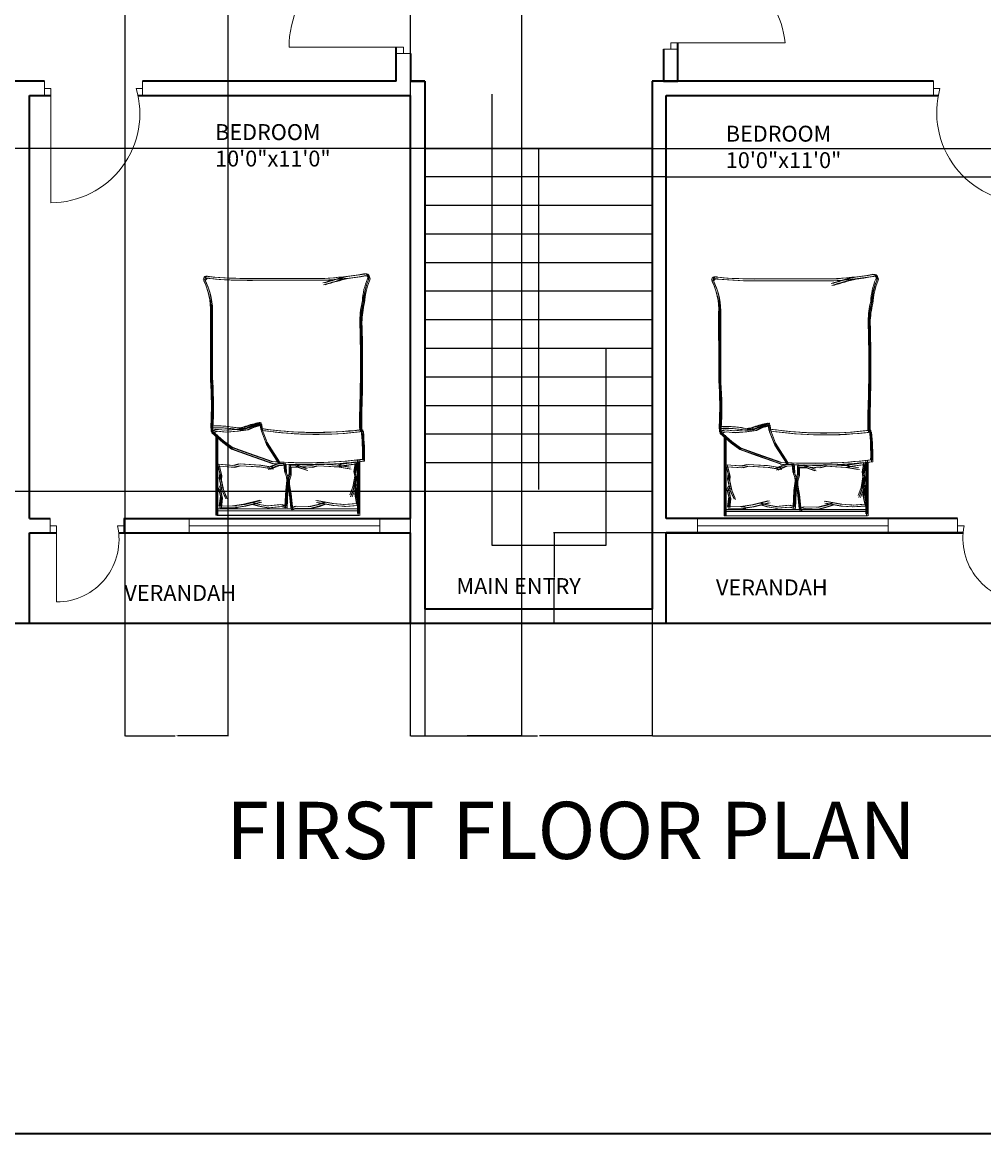
# Model space of a CAD drawing. Units: inches. Extents: x 2234 to 3001, y 1541 to 2386.
# Tile 2 of 12: x 2437 to 2739, y 1541 to 1891. Entities that reach past the tile are written whole.
import ezdxf

# ---------------------------------------------------------------- set-up
doc = ezdxf.new("R2010")
doc.units = ezdxf.units.IN
for name, color, linetype, lineweight in [('A-ANNO-DIMS', 2, 'Continuous', 18), ('A-ANNO-TEXT', 7, 'Continuous', 25), ('A-ANNO-TTLB', 7, 'Continuous', 35), ('A-AREA-IDEN', 7, 'Continuous', 18), ('A-DOOR', 3, 'Continuous', 18), ('A-FLOR-STRS', 7, 'Continuous', 25), ('A-FURN', 9, 'Continuous', 13), ('A-GLAZ', 4, 'Continuous', 18), ('A-WALL', 7, 'Continuous', 35)]:
    doc.layers.add(name, color=color, linetype=linetype, lineweight=lineweight)
doc.styles.get("Standard").update_dxf_attribs({"font": 'arial.ttf'})
doc.dimstyles.get("Standard").update_dxf_attribs({"dimtxt": 0.18, "dimasz": 0.18, "dimexe": 0.18, "dimexo": 0.0625, "dimgap": 0.09, "dimtad": 0, "dimtih": 1, "dimtoh": 1, "dimdec": 4, "dimzin": 0, "dimdsep": 46, "dimtxsty": 'Standard', "dimcen": 0.09, "dimadec": 0, "dimazin": 0, "dimtfac": 1, "dimtdec": 4, "dimtofl": 0, "dimtmove": 0, "dimatfit": 3, "dimfxl": 1, "dimtolj": 1, "dimtzin": 0, "dimarcsym": 0})

# ---------------------------------------------------------------- blocks, each defined once
blk = doc.blocks.new('WIN-60-A')
for p, q in [((0, 60), (4.5, 60)), ((4.5, 60), (2.25, 60)), ((2.25, 60), (2.25, 0)), ((2.25, 0), (0, 0)), ((0, 0), (4.5, 0))]:
    blk.add_line(p, q)
blk = doc.blocks.new('BED-DOUBLE-B')
for p, q in [((37.77, 74.61), (14.78, 74.61)), ((37.77, 74.61), (14.78, 74.61)), ((37.98, 74.02), (15, 74.02)), ((37.98, 74.02), (15, 74.02)), ((38.22, 74.59), (15.24, 74.59)), ((38.22, 74.59), (15.24, 74.59)), ((38.44, 73.99), (15.45, 73.99)), ((38.44, 73.99), (15.46, 73.99)), ((2.39, 28.15), (2.47, 26.53, 3.61)), ((2.39, 28.15), (2.47, 26.53, 3.61)), ((2.85, 28.13), (2.92, 26.5, 3.61)), ((2.85, 28.13), (2.93, 26.5, 3.61)), ((15.47, 28.4), (13.59, 27.54)), ((15.47, 28.4), (13.59, 27.54)), ((15.93, 28.38), (14.05, 27.52)), ((15.93, 28.38), (14.05, 27.52)), ((17.79, 28.98), (15.47, 28.4)), ((17.79, 28.98), (15.47, 28.4)), ((18, 28.38), (15.68, 27.81)), ((18, 28.38), (15.69, 27.81)), ((18.24, 28.96), (15.93, 28.38)), ((18.24, 28.96), (15.93, 28.38)), ((18.46, 28.36), (16.14, 27.79)), ((18.46, 28.36), (16.14, 27.79)), ((18.07, 27.1), (17.79, 28.98)), ((18.07, 27.1), (17.79, 28.98)), ((18.29, 26.51), (18, 28.38)), ((18.29, 26.51), (18, 28.38)), ((18.53, 27.08), (18.24, 28.96)), ((18.53, 27.08), (18.24, 28.96)), ((18.75, 26.49), (18.46, 28.36)), ((18.75, 26.49), (18.46, 28.36)), ((3.9, 27.1), (2.47, 26.53)), ((3.9, 27.1), (2.47, 26.53)), ((2.47, 26.53), (5.93, 23.49)), ((2.47, 26.53), (5.93, 23.49)), ((2.61, 27.56), (2.68, 25.93, 3.61)), ((2.61, 27.56), (2.68, 25.93, 3.61)), ((4.12, 26.51), (2.68, 25.93)), ((4.12, 26.51), (2.68, 25.93)), ((2.68, 25.93), (6.14, 22.89)), ((2.68, 25.93), (6.14, 22.89)), ((4.36, 27.08), (2.92, 26.5)), ((2.92, 26.5), (6.38, 23.47)), ((4.36, 27.08), (2.93, 26.5)), ((2.93, 26.5), (6.39, 23.47)), ((3.06, 27.54), (3.14, 25.91, 3.61)), ((3.06, 27.54), (3.14, 25.91, 3.61)), ((4.57, 26.49), (3.14, 25.91)), ((4.57, 26.49), (3.14, 25.91)), ((3.14, 25.91), (6.6, 22.87)), ((3.14, 25.91), (6.6, 22.87)), ((6.79, 26.81), (3.9, 27.1)), ((6.8, 26.81), (3.9, 27.1)), ((3.96, 0.62), (3.96, 25.46)), ((3.96, 0.62), (3.96, 25.46)), ((7.01, 26.22), (4.12, 26.51)), ((7.01, 26.22), (4.12, 26.51)), ((4.18, 0.02), (4.18, 24.87)), ((4.18, 0.02), (4.18, 24.87)), ((7.25, 26.79), (4.36, 27.08)), ((7.25, 26.79), (4.36, 27.08)), ((4.42, 0.6), (4.42, 25.44)), ((4.42, 0.6), (4.42, 25.44)), ((7.47, 26.2), (4.57, 26.49)), ((7.47, 26.2), (4.57, 26.49)), ((4.63, 0), (4.63, 24.85)), ((4.63, 0), (4.63, 24.85)), ((10.41, 27.1), (6.79, 26.81)), ((10.41, 27.1), (6.8, 26.81)), ((10.62, 26.51), (7.01, 26.22)), ((10.62, 26.51), (7.01, 26.22)), ((10.87, 27.08), (7.25, 26.79)), ((10.87, 27.08), (7.25, 26.79)), ((11.08, 26.49), (7.47, 26.2)), ((11.08, 26.49), (7.47, 26.2)), ((13.59, 27.54), (10.41, 27.1)), ((13.59, 27.54), (10.41, 27.1)), ((13.8, 26.94), (10.62, 26.51)), ((13.81, 26.94), (10.62, 26.51)), ((14.05, 27.52), (10.87, 27.08)), ((14.05, 27.52), (10.87, 27.08)), ((14.26, 26.92), (11.08, 26.49)), ((14.26, 26.92), (11.08, 26.49)), ((15.68, 27.81), (13.8, 26.94)), ((15.69, 27.81), (13.81, 26.94)), ((16.14, 27.79), (14.26, 26.92)), ((16.14, 27.79), (14.26, 26.92)), ((19.67, 22.91), (18.07, 27.1)), ((19.67, 22.91), (18.07, 27.1)), ((19.88, 22.32), (18.29, 26.51)), ((19.88, 22.32), (18.29, 26.51)), ((20.12, 22.89), (18.53, 27.08)), ((20.12, 22.89), (18.53, 27.08)), ((20.34, 22.29), (18.75, 26.49)), ((20.34, 22.29), (18.75, 26.49)), ((5.93, 23.49), (8.67, 21.47)), ((5.93, 23.49), (8.68, 21.47)), ((6.14, 22.89), (8.89, 20.87)), ((6.14, 22.89), (8.89, 20.87)), ((6.38, 23.47), (9.13, 21.45)), ((6.39, 23.47), (9.13, 21.45)), ((6.6, 22.87), (9.35, 20.85)), ((6.6, 22.87), (9.35, 20.85)), ((8.67, 21.47), (13.88, 19.59)), ((8.68, 21.47), (13.88, 19.59)), ((9.13, 21.45), (14.34, 19.57)), ((9.13, 21.45), (14.34, 19.57)), ((23.58, 16.85), (19.67, 22.91)), ((23.58, 16.85), (19.67, 22.91)), ((23.79, 16.25), (19.88, 22.32)), ((23.79, 16.25), (19.88, 22.32)), ((24.04, 16.83), (20.12, 22.89)), ((24.04, 16.83), (20.12, 22.89)), ((24.25, 16.23), (20.34, 22.29)), ((24.25, 16.23), (20.34, 22.29)), ((8.89, 20.87), (14.09, 18.99)), ((8.89, 20.87), (14.09, 18.99)), ((9.35, 20.85), (14.55, 18.97)), ((9.35, 20.85), (14.55, 18.97)), ((13.88, 19.59), (21.67, 16.85)), ((13.88, 19.59), (21.67, 16.85)), ((14.09, 18.99), (21.88, 16.25)), ((14.09, 18.99), (21.88, 16.25)), ((14.34, 19.57), (22.12, 16.83)), ((14.34, 19.57), (22.12, 16.83)), ((14.55, 18.97), (22.34, 16.23)), ((14.55, 18.97), (22.34, 16.23)), ((48.59, 17.53), (48.59, 0.62)), ((48.59, 17.53), (48.59, 0.62)), ((49.05, 17.51), (49.05, 0.6)), ((49.05, 17.51), (49.05, 0.6)), ((9.28, 15.72), (4.49, 16.09)), ((4.49, 16.09), (5.22, 13.16)), ((9.29, 15.72), (4.49, 16.09)), ((4.49, 16.09), (5.22, 13.16)), ((9.5, 15.12), (4.71, 15.5)), ((4.71, 15.5), (5.43, 12.56)), ((9.5, 15.12), (4.71, 15.5)), ((4.71, 15.5), (5.43, 12.56)), ((9.74, 15.69), (4.95, 16.07)), ((4.95, 16.07), (5.67, 13.14)), ((9.74, 15.69), (4.95, 16.07)), ((4.95, 16.07), (5.67, 13.14)), ((9.96, 15.1), (5.16, 15.47)), ((5.16, 15.47), (5.89, 12.54)), ((9.96, 15.1), (5.16, 15.47)), ((5.16, 15.47), (5.89, 12.54)), ((11.12, 16.24), (9.28, 15.72)), ((11.12, 16.24), (9.29, 15.72)), ((11.33, 15.64), (9.5, 15.12)), ((11.33, 15.64), (9.5, 15.12)), ((11.57, 16.21), (9.74, 15.69)), ((11.57, 16.21), (9.74, 15.69)), ((11.79, 15.62), (9.96, 15.1)), ((11.79, 15.62), (9.96, 15.1)), ((17.66, 15.83), (11.12, 16.24)), ((17.66, 15.83), (11.12, 16.24)), ((17.87, 15.24), (11.33, 15.64)), ((17.87, 15.24), (11.33, 15.64)), ((18.12, 15.81), (11.57, 16.21)), ((18.12, 15.81), (11.57, 16.21)), ((18.33, 15.22), (11.79, 15.62)), ((18.33, 15.22), (11.79, 15.62)), ((21.43, 15.21), (17.66, 15.83)), ((21.43, 15.21), (17.66, 15.83)), ((21.64, 14.61), (17.87, 15.24)), ((21.64, 14.61), (17.87, 15.24)), ((21.88, 15.19), (18.12, 15.81)), ((21.88, 15.19), (18.12, 15.81)), ((22.1, 14.59), (18.33, 15.22)), ((22.1, 14.59), (18.33, 15.22)), ((23.12, 16.25), (20.25, 15.05)), ((23.12, 16.25), (20.25, 15.05)), ((23.33, 15.65), (20.47, 14.45)), ((23.33, 15.65), (20.47, 14.45)), ((23.58, 16.23), (20.71, 15.03)), ((23.58, 16.23), (20.71, 15.03)), ((23.79, 15.63), (20.92, 14.43)), ((23.79, 15.63), (20.92, 14.43)), ((25.41, 16.39), (23.12, 16.25)), ((25.41, 16.39), (23.12, 16.25)), ((25.62, 15.79), (23.33, 15.65)), ((25.62, 15.79), (23.33, 15.65)), ((25.87, 16.37), (23.58, 16.23)), ((25.87, 16.37), (23.58, 16.23)), ((26.08, 15.77), (23.79, 15.63)), ((26.08, 15.77), (23.79, 15.63)), ((25.57, 13.89), (25.41, 16.39)), ((25.57, 13.89), (25.41, 16.39)), ((25.78, 13.3), (25.62, 15.79)), ((25.78, 13.3), (25.62, 15.79)), ((26.02, 13.87), (25.87, 16.37)), ((26.02, 13.87), (25.87, 16.37)), ((26.24, 13.27), (26.08, 15.77)), ((26.24, 13.27), (26.08, 15.77)), ((27.03, 13.3), (27.03, 15.8)), ((27.03, 15.8), (29.33, 15.8)), ((27.03, 13.3), (27.03, 15.8)), ((27.03, 15.8), (29.33, 15.8)), ((27.24, 12.7), (27.24, 15.21)), ((27.24, 15.21), (29.54, 15.21)), ((27.24, 12.7), (27.24, 15.21)), ((27.24, 15.21), (29.54, 15.21)), ((27.49, 13.28), (27.49, 15.78)), ((27.49, 15.78), (29.78, 15.78)), ((27.49, 13.28), (27.49, 15.78)), ((27.49, 15.78), (29.78, 15.78)), ((27.7, 12.68), (27.7, 15.19)), ((27.7, 15.19), (30, 15.19)), ((27.7, 12.68), (27.7, 15.19)), ((27.7, 15.19), (30, 15.19)), ((33.73, 15.72), (28.94, 16.09)), ((33.73, 15.72), (28.94, 16.09)), ((33.95, 15.12), (29.15, 15.5)), ((33.95, 15.12), (29.15, 15.5)), ((29.33, 15.8), (32.26, 14.78)), ((29.33, 15.8), (32.26, 14.78)), ((34.19, 15.69), (29.4, 16.07)), ((34.19, 15.69), (29.4, 16.07)), ((29.54, 15.21), (32.48, 14.19)), ((29.54, 15.21), (32.48, 14.19)), ((34.4, 15.1), (29.61, 15.47)), ((34.4, 15.1), (29.61, 15.47)), ((29.78, 15.78), (32.72, 14.76)), ((29.78, 15.78), (32.72, 14.76)), ((30, 15.19), (32.93, 14.17)), ((30, 15.19), (32.93, 14.17)), ((35.56, 16.24), (33.73, 15.72)), ((35.56, 16.24), (33.73, 15.72)), ((35.78, 15.64), (33.95, 15.12)), ((35.78, 15.64), (33.95, 15.12)), ((36.02, 16.21), (34.19, 15.69)), ((36.02, 16.21), (34.19, 15.69)), ((36.23, 15.62), (34.4, 15.1)), ((36.23, 15.62), (34.4, 15.1)), ((42.11, 15.83), (35.56, 16.24)), ((42.11, 15.83), (35.56, 16.24)), ((42.32, 15.24), (35.78, 15.64)), ((42.32, 15.24), (35.78, 15.64)), ((42.57, 15.81), (36.02, 16.21)), ((42.57, 15.81), (36.02, 16.21)), ((42.78, 15.22), (36.23, 15.62)), ((42.78, 15.22), (36.23, 15.62)), ((42.11, 15.83), (43.17, 16.13)), ((42.11, 15.83), (43.17, 16.13)), ((45.87, 15.21), (42.11, 15.83)), ((45.87, 15.21), (42.11, 15.83)), ((42.32, 15.24), (43.38, 15.54)), ((42.32, 15.24), (43.38, 15.54)), ((46.09, 14.61), (42.32, 15.24)), ((46.09, 14.61), (42.32, 15.24)), ((42.57, 15.81), (43.62, 16.11)), ((42.57, 15.81), (43.62, 16.11)), ((46.33, 15.19), (42.57, 15.81)), ((46.33, 15.19), (42.57, 15.81)), ((42.78, 15.22), (43.84, 15.52)), ((42.78, 15.22), (43.84, 15.52)), ((46.54, 14.59), (42.78, 15.22)), ((46.54, 14.59), (42.78, 15.22)), ((43.17, 16.13), (47.93, 16.81)), ((43.17, 16.13), (47.93, 16.81)), ((43.38, 15.54), (48.14, 16.21)), ((43.38, 15.54), (48.14, 16.21)), ((43.62, 16.11), (48.38, 16.79)), ((43.62, 16.11), (48.38, 16.79)), ((43.84, 15.52), (48.6, 16.19)), ((43.84, 15.52), (48.6, 16.19)), ((47.93, 16.81), (47.39, 13.84)), ((47.93, 16.81), (47.39, 13.84)), ((48.14, 16.21), (47.6, 13.24)), ((48.14, 16.21), (47.6, 13.24)), ((48.38, 16.79), (47.84, 13.82)), ((48.38, 16.79), (47.84, 13.82)), ((48.6, 16.19), (48.06, 13.22)), ((48.6, 16.19), (48.06, 13.22)), ((48.8, 16.93), (48.8, 0.02)), ((48.8, 16.93), (48.8, 0.02)), ((49.26, 16.91), (49.26, 0)), ((49.26, 16.91), (49.26, 0)), ((5.22, 13.16), (5.04, 11.66)), ((5.22, 13.16), (5.04, 11.66)), ((5.04, 11.66), (5.79, 8.33)), ((5.04, 11.66), (5.79, 8.33)), ((5.43, 12.56), (5.25, 11.07)), ((5.43, 12.56), (5.25, 11.07)), ((5.25, 11.07), (6, 7.73)), ((5.25, 11.07), (6, 7.73)), ((5.67, 13.14), (5.5, 11.64)), ((5.67, 13.14), (5.5, 11.64)), ((5.5, 11.64), (6.25, 8.31)), ((5.5, 11.64), (6.25, 8.31)), ((5.89, 12.54), (5.71, 11.04)), ((5.89, 12.54), (5.71, 11.04)), ((5.71, 11.04), (6.46, 7.71)), ((5.71, 11.04), (6.46, 7.71)), ((26.21, 12.17), (25.57, 13.89)), ((26.21, 12.17), (25.57, 13.89)), ((26.43, 11.58), (25.78, 13.3)), ((26.43, 11.58), (25.78, 13.3)), ((25.94, 7.96), (26.29, 10.96)), ((25.94, 7.96), (26.29, 10.96)), ((26.67, 12.15), (26.02, 13.87)), ((26.67, 12.15), (26.02, 13.87)), ((26.29, 10.96), (26.21, 12.17)), ((26.29, 10.96), (26.21, 12.17)), ((26.88, 11.56), (26.24, 13.27)), ((26.89, 11.56), (26.24, 13.27)), ((26.39, 7.94), (26.75, 10.94)), ((26.39, 7.94), (26.75, 10.94)), ((26.5, 10.36), (26.43, 11.58)), ((26.5, 10.36), (26.43, 11.58)), ((26.49, 11.54), (27.03, 13.3)), ((26.49, 11.54), (27.03, 13.3)), ((26.49, 10.33), (26.49, 11.54)), ((26.49, 10.33), (26.49, 11.54)), ((26.75, 10.94), (26.67, 12.15)), ((26.75, 10.94), (26.67, 12.15)), ((26.7, 10.95), (27.24, 12.7)), ((26.7, 10.95), (27.24, 12.7)), ((26.7, 9.73), (26.7, 10.95)), ((26.7, 9.73), (26.7, 10.95)), ((26.96, 10.34), (26.88, 11.56)), ((26.96, 10.34), (26.89, 11.56)), ((26.95, 11.52), (27.49, 13.28)), ((26.95, 11.52), (27.49, 13.28)), ((26.95, 10.31), (26.95, 11.52)), ((26.95, 10.31), (26.95, 11.52)), ((27.16, 10.93), (27.7, 12.68)), ((27.16, 10.93), (27.7, 12.68)), ((27.16, 9.71), (27.16, 10.93)), ((27.16, 9.71), (27.16, 10.93)), ((47.66, 12.35), (47.12, 8.98)), ((47.66, 12.35), (47.12, 8.98)), ((47.87, 11.76), (47.33, 8.38)), ((47.87, 11.76), (47.33, 8.38)), ((47.39, 13.84), (47.66, 12.35)), ((47.39, 13.84), (47.66, 12.35)), ((48.11, 12.33), (47.57, 8.96)), ((48.11, 12.33), (47.57, 8.96)), ((47.6, 13.24), (47.87, 11.76)), ((47.6, 13.24), (47.87, 11.76)), ((48.33, 11.74), (47.79, 8.36)), ((48.33, 11.74), (47.79, 8.36)), ((47.84, 13.82), (48.11, 12.33)), ((47.84, 13.82), (48.11, 12.33)), ((48.06, 13.22), (48.33, 11.74)), ((48.06, 13.22), (48.33, 11.74)), ((4.84, 8.4), (5.32, 9.38)), ((4.84, 8.4), (5.32, 9.38)), ((5.39, 6), (4.84, 8.4)), ((5.39, 6), (4.84, 8.4)), ((5.05, 7.81), (5.53, 8.78)), ((5.05, 7.81), (5.53, 8.78)), ((5.61, 5.41), (5.05, 7.81)), ((5.61, 5.41), (5.05, 7.81)), ((5.3, 8.38), (5.78, 9.36)), ((5.3, 8.38), (5.78, 9.36)), ((5.85, 5.98), (5.3, 8.38)), ((5.85, 5.98), (5.3, 8.38)), ((5.51, 7.79), (5.99, 8.76)), ((5.51, 7.79), (5.99, 8.76)), ((6.06, 5.39), (5.51, 7.79)), ((6.07, 5.39), (5.51, 7.79)), ((5.79, 8.33), (6.89, 5.83)), ((5.79, 8.33), (6.89, 5.83)), ((6, 7.73), (7.11, 5.23)), ((6, 7.73), (7.11, 5.23)), ((6.25, 8.31), (7.35, 5.81)), ((6.25, 8.31), (7.35, 5.81)), ((6.46, 7.71), (7.56, 5.21)), ((6.46, 7.71), (7.56, 5.21)), ((25.71, 2.94), (25.94, 7.96)), ((25.71, 2.94), (25.94, 7.96)), ((25.92, 2.35), (26.15, 7.37)), ((25.92, 2.35), (26.15, 7.37)), ((26.15, 7.37), (26.5, 10.36)), ((26.15, 7.37), (26.5, 10.36)), ((26.17, 2.92), (26.39, 7.94)), ((26.17, 2.92), (26.39, 7.94)), ((26.38, 2.33), (26.61, 7.35)), ((26.38, 2.33), (26.61, 7.35)), ((27.03, 7.36), (26.49, 10.33)), ((27.03, 7.36), (26.49, 10.33)), ((26.61, 7.35), (26.96, 10.34)), ((26.61, 7.35), (26.96, 10.34)), ((27.24, 6.76), (26.7, 9.73)), ((27.24, 6.76), (26.7, 9.73)), ((27.49, 7.34), (26.95, 10.31)), ((27.49, 7.34), (26.95, 10.31)), ((27.57, 2.36), (27.03, 7.36)), ((27.57, 2.36), (27.03, 7.36)), ((27.7, 6.74), (27.16, 9.71)), ((27.7, 6.74), (27.16, 9.71)), ((28.03, 2.34), (27.49, 7.34)), ((28.03, 2.34), (27.49, 7.34)), ((47.12, 8.98), (46.17, 6.41)), ((47.12, 8.98), (46.17, 6.41)), ((47.33, 8.38), (46.38, 5.82)), ((47.33, 8.38), (46.38, 5.82)), ((47.57, 8.96), (46.63, 6.39)), ((47.57, 8.96), (46.63, 6.39)), ((47.79, 8.36), (46.84, 5.8)), ((47.79, 8.36), (46.84, 5.8)), ((48.06, 9.11), (47.52, 10.06)), ((48.06, 9.11), (47.52, 10.06)), ((47.66, 6.68), (48.06, 9.11)), ((47.66, 6.68), (48.06, 9.11)), ((48.27, 8.52), (47.73, 9.46)), ((48.27, 8.52), (47.73, 9.46)), ((47.87, 6.09), (48.27, 8.52)), ((47.87, 6.09), (48.27, 8.52)), ((48.52, 9.09), (47.98, 10.04)), ((48.52, 9.09), (47.98, 10.04)), ((48.11, 6.66), (48.52, 9.09)), ((48.11, 6.66), (48.52, 9.09)), ((48.73, 8.5), (48.19, 9.44)), ((48.73, 8.5), (48.19, 9.44)), ((48.33, 6.07), (48.73, 8.5)), ((48.33, 6.07), (48.73, 8.5)), ((5.04, 3.01), (5.39, 6)), ((5.04, 3.01), (5.39, 6)), ((5.25, 2.41), (5.61, 5.41)), ((5.25, 2.41), (5.61, 5.41)), ((5.5, 2.98), (5.85, 5.98)), ((5.5, 2.98), (5.85, 5.98)), ((5.71, 2.39), (6.06, 5.39)), ((5.71, 2.39), (6.07, 5.39)), ((12.69, 3.48), (17.76, 4.75)), ((12.7, 3.48), (17.76, 4.75)), ((12.91, 2.89), (17.97, 4.15)), ((12.91, 2.89), (17.97, 4.15)), ((13.15, 3.46), (18.21, 4.73)), ((13.15, 3.46), (18.21, 4.73)), ((13.37, 2.87), (18.43, 4.13)), ((13.37, 2.87), (18.43, 4.13)), ((15.23, 4.05), (17.16, 3.49)), ((15.23, 4.05), (17.16, 3.49)), ((15.69, 4.03), (17.61, 3.47)), ((15.69, 4.03), (17.62, 3.47)), ((27.78, 1.77), (27.24, 6.76)), ((27.78, 1.77), (27.24, 6.76)), ((28.24, 1.75), (27.7, 6.74)), ((28.24, 1.75), (27.7, 6.74)), ((40.53, 3.71), (35.4, 4.66)), ((40.53, 3.71), (35.4, 4.66)), ((40.74, 3.12), (35.61, 4.06)), ((40.74, 3.12), (35.61, 4.06)), ((40.98, 3.69), (35.85, 4.64)), ((40.98, 3.69), (35.85, 4.64)), ((37.96, 4.12), (36.07, 3.44)), ((37.96, 4.12), (36.07, 3.44)), ((41.2, 3.1), (36.07, 4.04)), ((41.2, 3.1), (36.07, 4.04)), ((38.17, 3.52), (36.29, 2.85)), ((38.18, 3.52), (36.29, 2.85)), ((38.42, 4.1), (36.53, 3.42)), ((38.42, 4.1), (36.53, 3.42)), ((38.63, 3.5), (36.74, 2.83)), ((38.63, 3.5), (36.74, 2.83)), ((44.1, 3.44), (40.53, 3.71)), ((44.1, 3.44), (40.53, 3.71)), ((44.55, 3.42), (40.98, 3.69)), ((44.55, 3.42), (40.98, 3.69)), ((48.19, 3.73), (44.19, 3.43)), ((48.19, 3.73), (44.2, 3.43)), ((48.65, 3.71), (44.65, 3.41)), ((48.65, 3.71), (44.65, 3.41)), ((48.2, 3.71), (47.66, 6.68)), ((48.2, 3.71), (47.66, 6.68)), ((48.41, 3.12), (47.87, 6.09)), ((48.41, 3.12), (47.87, 6.09)), ((48.65, 3.69), (48.11, 6.66)), ((48.65, 3.69), (48.11, 6.66)), ((48.87, 3.1), (48.33, 6.07)), ((48.87, 3.1), (48.33, 6.07)), ((48.59, 2.05), (3.96, 2.05)), ((48.59, 2.05), (3.96, 2.05)), ((3.96, 0.02), (3.96, 0.62)), ((3.96, 0.02), (48.59, 0.02)), ((48.8, 1.45), (4.18, 1.45)), ((48.8, 1.45), (4.18, 1.45)), ((49.05, 2.03), (4.42, 2.03)), ((49.05, 2.03), (4.42, 2.03)), ((4.42, 0), (4.42, 0.6)), ((49.26, 1.43), (4.63, 1.43)), ((49.26, 1.43), (4.63, 1.43)), ((5.04, 3.01), (10.08, 2.91)), ((5.04, 3.01), (10.09, 2.91)), ((5.25, 2.41), (10.3, 2.32)), ((5.25, 2.41), (10.3, 2.32)), ((5.5, 2.98), (10.54, 2.89)), ((5.5, 2.98), (10.54, 2.89)), ((5.71, 2.39), (10.76, 2.3)), ((5.71, 2.39), (10.76, 2.3)), ((9.15, 2.99), (12.69, 3.48)), ((9.15, 2.99), (12.7, 3.48)), ((10.08, 2.91), (9.15, 2.99)), ((10.09, 2.91), (9.15, 2.99)), ((9.36, 2.39), (12.91, 2.89)), ((9.36, 2.39), (12.91, 2.89)), ((10.3, 2.32), (9.36, 2.39)), ((10.3, 2.32), (9.36, 2.39)), ((9.61, 2.97), (13.15, 3.46)), ((9.61, 2.97), (13.15, 3.46)), ((10.54, 2.89), (9.61, 2.97)), ((10.54, 2.89), (9.61, 2.97)), ((9.82, 2.37), (13.37, 2.87)), ((9.82, 2.37), (13.37, 2.87)), ((10.76, 2.3), (9.82, 2.37)), ((10.76, 2.3), (9.82, 2.37)), ((15.44, 3.45), (17.37, 2.89)), ((15.44, 3.45), (17.37, 2.89)), ((15.9, 3.43), (17.83, 2.87)), ((15.9, 3.43), (17.83, 2.87)), ((17.16, 3.49), (19.89, 2.99)), ((17.16, 3.49), (19.89, 2.99)), ((17.37, 2.89), (20.11, 2.39)), ((17.37, 2.89), (20.11, 2.39)), ((17.61, 3.47), (20.35, 2.97)), ((17.62, 3.47), (20.35, 2.97)), ((17.83, 2.87), (20.56, 2.37)), ((17.83, 2.87), (20.56, 2.37)), ((19.89, 2.99), (20.19, 3.01)), ((19.89, 2.99), (20.19, 3.01)), ((20.11, 2.39), (20.41, 2.41)), ((20.11, 2.39), (20.41, 2.41)), ((20.19, 3.01), (24.33, 3.4)), ((20.19, 3.01), (24.33, 3.4)), ((20.35, 2.97), (20.65, 2.98)), ((20.35, 2.97), (20.65, 2.98)), ((20.41, 2.41), (24.54, 2.8)), ((20.41, 2.41), (24.54, 2.8)), ((20.56, 2.37), (20.86, 2.39)), ((20.56, 2.37), (20.86, 2.39)), ((20.65, 2.98), (24.79, 3.38)), ((20.65, 2.98), (24.79, 3.38)), ((20.86, 2.39), (25, 2.78)), ((20.86, 2.39), (25, 2.78)), ((24.33, 3.4), (25.71, 2.94)), ((24.33, 3.4), (25.71, 2.94)), ((24.54, 2.8), (25.92, 2.35)), ((24.54, 2.8), (25.92, 2.35)), ((24.79, 3.38), (26.17, 2.92)), ((24.79, 3.38), (26.17, 2.92)), ((25, 2.78), (26.38, 2.33)), ((25, 2.78), (26.38, 2.33)), ((28.92, 2.9), (27.57, 2.36)), ((28.92, 2.9), (27.57, 2.36)), ((29.13, 2.31), (27.78, 1.77)), ((29.13, 2.31), (27.78, 1.77)), ((29.38, 2.88), (28.03, 2.34)), ((29.38, 2.88), (28.03, 2.34)), ((29.59, 2.29), (28.24, 1.75)), ((29.59, 2.29), (28.24, 1.75)), ((33.07, 2.77), (28.92, 2.9)), ((33.07, 2.77), (28.92, 2.9)), ((33.29, 2.17), (29.13, 2.31)), ((33.29, 2.17), (29.13, 2.31)), ((33.53, 2.75), (29.38, 2.88)), ((33.53, 2.75), (29.38, 2.88)), ((33.74, 2.15), (29.59, 2.29)), ((33.74, 2.15), (29.59, 2.29)), ((33.37, 2.77), (33.07, 2.77)), ((33.37, 2.77), (33.07, 2.77)), ((33.59, 2.17), (33.29, 2.17)), ((33.59, 2.17), (33.29, 2.17)), ((36.07, 3.44), (33.37, 2.77)), ((36.07, 3.44), (33.37, 2.77)), ((33.83, 2.75), (33.53, 2.75)), ((33.83, 2.75), (33.53, 2.75)), ((36.29, 2.85), (33.59, 2.17)), ((36.29, 2.85), (33.59, 2.17)), ((34.04, 2.15), (33.74, 2.15)), ((34.04, 2.15), (33.74, 2.15)), ((36.53, 3.42), (33.83, 2.75)), ((36.53, 3.42), (33.83, 2.75)), ((36.74, 2.83), (34.04, 2.15)), ((36.74, 2.83), (34.04, 2.15)), ((44.31, 2.85), (40.74, 3.12)), ((44.31, 2.85), (40.74, 3.12)), ((44.77, 2.83), (41.2, 3.1)), ((44.77, 2.83), (41.2, 3.1)), ((44.19, 3.43), (44.1, 3.44)), ((44.2, 3.43), (44.1, 3.44)), ((44.41, 2.83), (44.31, 2.85)), ((44.41, 2.83), (44.31, 2.85)), ((48.41, 3.14), (44.41, 2.83)), ((48.41, 3.14), (44.41, 2.83)), ((44.65, 3.41), (44.55, 3.42)), ((44.65, 3.41), (44.55, 3.42)), ((44.87, 2.81), (44.77, 2.83)), ((44.87, 2.81), (44.77, 2.83)), ((48.86, 3.12), (44.87, 2.81)), ((48.86, 3.12), (44.87, 2.81)), ((4.42, 0), (49.05, 0))]:
    blk.add_line(p, q)
for centre, radius, start, end in [((1.03, 74.26), 1.03, 62.6588, 176.02), ((1.03, 74.26), 1.03, 62.6588, 176.02), ((-19.28, 64.73), 21.54, 357.4714, 26.4681), ((-19.28, 64.73), 21.54, 357.4714, 26.4681), ((1.24, 73.67), 1.03, 62.6588, 176.02), ((1.24, 73.67), 1.03, 62.6588, 176.02), ((-19.07, 64.14), 21.54, 357.4714, 26.4681), ((-19.07, 64.14), 21.54, 357.4714, 26.4681), ((1.48, 74.24), 1.03, 62.6588, 176.02), ((1.49, 74.24), 1.03, 62.6588, 176.02), ((-18.82, 64.71), 21.54, 357.4714, 26.4681), ((-18.82, 64.71), 21.54, 357.4714, 26.4681), ((1.7, 73.64), 1.03, 62.6588, 176.02), ((1.7, 73.64), 1.03, 62.6588, 176.02), ((-18.61, 64.12), 21.54, 357.4714, 26.4681), ((-18.61, 64.12), 21.54, 357.4714, 26.4681), ((13.41, 198.83), 124.23, 264.4998, 270.6351), ((13.41, 198.83), 124.23, 264.4998, 270.6351), ((13.62, 198.23), 124.23, 264.4998, 270.6351), ((13.62, 198.23), 124.23, 264.4998, 270.6351), ((13.86, 198.81), 124.23, 264.4998, 270.6351), ((13.86, 198.81), 124.23, 264.4998, 270.6351), ((14.08, 198.21), 124.23, 264.4998, 270.6351), ((14.08, 198.21), 124.23, 264.4998, 270.6351), ((67.91, -21.52), 99.41, 103.3832, 107.7053), ((67.91, -21.52), 99.41, 103.3832, 107.7053), ((31.83, 188.15), 113.69, 272.9958, 279.4091), ((31.83, 188.15), 113.69, 272.9958, 279.4091), ((68.13, -22.12), 99.41, 103.3832, 107.7053), ((68.13, -22.12), 99.41, 103.3832, 107.7053), ((32.04, 187.55), 113.69, 272.9958, 279.4091), ((32.04, 187.55), 113.69, 272.9958, 279.4091), ((68.37, -21.54), 99.41, 103.3832, 107.7053), ((68.37, -21.54), 99.41, 103.3832, 107.7053), ((32.28, 188.13), 113.69, 272.9958, 279.4091), ((32.28, 188.13), 113.69, 272.9958, 279.4091), ((68.58, -22.14), 99.41, 103.3832, 107.7053), ((68.58, -22.14), 99.41, 103.3832, 107.7053), ((32.5, 187.53), 113.69, 272.9958, 279.4091), ((32.5, 187.53), 113.69, 272.9958, 279.4091), ((72.06, 66.24), 22, 157.9751, 176.652), ((72.06, 66.24), 22, 157.9751, 176.652), ((72.27, 65.64), 22, 157.9751, 176.652), ((72.27, 65.64), 22, 157.9751, 176.652), ((50.82, 75.05), 1.02, 326.1736, 113.4781), ((50.82, 75.05), 1.02, 326.1736, 113.4781), ((72.51, 66.22), 22, 157.9751, 176.652), ((72.51, 66.22), 22, 157.9751, 176.652), ((51.03, 74.46), 1.02, 326.1736, 113.4781), ((51.03, 74.46), 1.02, 326.1736, 113.4781), ((72.73, 65.62), 22, 157.9751, 176.652), ((72.73, 65.62), 22, 157.9751, 176.652), ((51.27, 75.03), 1.02, 326.1736, 113.4781), ((51.27, 75.03), 1.02, 326.1736, 113.4781), ((51.49, 74.44), 1.02, 326.1736, 113.4781), ((51.49, 74.44), 1.02, 326.1736, 113.4781), ((76.95, 60.86), 27.67, 166.0648, 178.9113), ((76.95, 60.86), 27.67, 166.0648, 178.9113), ((77.16, 60.26), 27.67, 166.0648, 178.9113), ((77.16, 60.26), 27.67, 166.0648, 178.9113), ((77.41, 60.84), 27.67, 166.0648, 178.9113), ((77.41, 60.84), 27.67, 166.0648, 178.9113), ((77.62, 60.24), 27.67, 166.0648, 178.9113), ((77.62, 60.24), 27.67, 166.0648, 178.9113), ((4261.85, 63.95), 4259.62, 180.00217, 180.28689), ((4261.85, 63.95), 4259.62, 180.00217, 180.28689), ((4262.07, 63.35), 4259.62, 180.00217, 180.28689), ((4262.07, 63.35), 4259.62, 180.00217, 180.28689), ((4262.31, 63.92), 4259.62, 180.00217, 180.28689), ((4262.31, 63.92), 4259.62, 180.00217, 180.28689), ((4262.53, 63.33), 4259.62, 180.00217, 180.28689), ((4262.53, 63.33), 4259.62, 180.00217, 180.28689), ((-400.87, 47.88), 450.36, 358.2277, 1.7185), ((-400.87, 47.88), 450.36, 358.2277, 1.7185), ((-400.66, 47.28), 450.36, 358.2277, 1.7185), ((-400.66, 47.28), 450.36, 358.2277, 1.7185), ((-400.41, 47.86), 450.36, 358.2277, 1.7185), ((-400.41, 47.86), 450.36, 358.2277, 1.7185), ((-400.2, 47.26), 450.36, 358.2277, 1.7185), ((-400.2, 47.26), 450.36, 358.2277, 1.7185), ((-118.36, 34.53), 120.92, 356.9791, 3.8365), ((-118.36, 34.53), 120.92, 356.9791, 3.8365), ((-118.14, 33.93), 120.92, 356.9791, 3.8365), ((-118.14, 33.93), 120.92, 356.9791, 3.8365), ((-117.9, 34.51), 120.92, 356.9791, 3.8365), ((-117.9, 34.51), 120.92, 356.9791, 3.8365), ((-117.69, 33.91), 120.92, 356.9791, 3.8365), ((-117.69, 33.91), 120.92, 356.9791, 3.8365), ((208.05, 29.73), 158.84, 178.4762, 181.0082), ((208.06, 29.73), 158.84, 178.4762, 181.0082), ((208.27, 29.13), 158.84, 178.4762, 181.0082), ((208.27, 29.13), 158.84, 178.4762, 181.0082), ((208.51, 29.7), 158.84, 178.4762, 181.0082), ((208.51, 29.7), 158.84, 178.4762, 181.0082), ((208.73, 29.11), 158.84, 178.4762, 181.0082), ((208.73, 29.11), 158.84, 178.4762, 181.0082), ((3.91, -5.6), 33.79, 79.8763, 92.5657), ((3.91, -5.6), 33.79, 79.8763, 92.5657), ((4.36, -5.62), 33.79, 79.8763, 92.5657), ((4.36, -5.62), 33.79, 79.8763, 92.5657), ((10.99, 33.36), 5.81, 258.6608, 293.7384), ((10.99, 33.36), 5.81, 258.6608, 293.7384), ((11.44, 33.34), 5.81, 258.6608, 293.7384), ((11.44, 33.34), 5.81, 258.6608, 293.7384), ((22.74, 2), 27.69, 100.6617, 109.8806), ((22.74, 2), 27.69, 100.6617, 109.8806), ((22.96, 1.4), 27.69, 100.6617, 109.8806), ((22.96, 1.4), 27.69, 100.6617, 109.8806), ((23.2, 1.98), 27.69, 100.6617, 109.8806), ((23.2, 1.98), 27.69, 100.6617, 109.8806), ((23.41, 1.38), 27.69, 100.6617, 109.8806), ((23.41, 1.38), 27.69, 100.6617, 109.8806), ((17.62, 29.04), 0.172, 340.2464, 91.1377), ((17.62, 29.04), 0.172, 340.2464, 91.1377), ((17.84, 28.44), 0.172, 340.2464, 91.1377), ((17.84, 28.44), 0.172, 340.2464, 91.1377), ((18.08, 29.02), 0.172, 340.2464, 91.1377), ((18.08, 29.02), 0.172, 340.2464, 91.1377), ((18.29, 28.42), 0.172, 340.2464, 91.1377), ((18.29, 28.42), 0.172, 340.2464, 91.1377), ((4.12, -6.19), 33.79, 79.8763, 92.5657), ((4.12, -6.19), 33.79, 79.8763, 92.5657), ((4.58, -6.22), 33.79, 79.8763, 92.5657), ((4.58, -6.22), 33.79, 79.8763, 92.5657), ((11.2, 32.76), 5.81, 258.6608, 293.7384), ((11.2, 32.76), 5.81, 258.6608, 293.7384), ((11.66, 32.74), 5.81, 258.6608, 293.7384), ((11.66, 32.74), 5.81, 258.6608, 293.7384), ((35.25, 146.58), 120.47, 261.7845, 276.9006), ((35.25, 146.58), 120.47, 261.7845, 276.9006), ((35.47, 145.98), 120.47, 261.7845, 276.9006), ((35.47, 145.98), 120.47, 261.7845, 276.9006), ((35.71, 146.56), 120.47, 261.7845, 276.9006), ((35.71, 146.56), 120.47, 261.7845, 276.9006), ((35.92, 145.96), 120.47, 261.7845, 276.9006), ((35.92, 145.96), 120.47, 261.7845, 276.9006), ((-27.69, 19.38), 77.79, 358.7218, 5.604), ((-27.69, 19.38), 77.79, 358.7218, 5.604), ((-27.47, 18.79), 77.79, 358.7218, 5.604), ((-27.47, 18.79), 77.79, 358.7218, 5.604), ((-27.23, 19.36), 77.79, 358.7218, 5.604), ((-27.23, 19.36), 77.79, 358.7218, 5.604), ((-27.02, 18.76), 77.79, 358.7218, 5.604), ((-27.02, 18.76), 77.79, 358.7218, 5.604), ((31.89, 170.61), 154.04, 266.0865, 276.7821), ((31.89, 170.61), 154.04, 266.0865, 276.7821), ((32.35, 170.59), 154.04, 266.0865, 276.7821), ((32.35, 170.59), 154.04, 266.0865, 276.7821), ((32.1, 170.01), 154.04, 266.0865, 276.7821), ((32.1, 170.01), 154.04, 266.0865, 276.7821), ((32.56, 169.99), 154.04, 266.0865, 276.7821), ((32.56, 169.99), 154.04, 266.0865, 276.7821)]:
    blk.add_arc(centre, radius, start, end)
blk = doc.blocks.new('*D64')
at = {"layer": 'A-ANNO-DIMS', "color": 0, "lineweight": -2, "transparency": 16777216}
for p, q in [((2563.25, 1706.55), (2563.25, 1666.58)), ((2634.75, 1706.55), (2634.75, 1666.58)), ((2563.43, 1666.76), (2598.68, 1666.76)), ((2634.57, 1666.76), (2599.33, 1666.76))]:
    blk.add_line(p, q, dxfattribs=at)
at = {"layer": 'A-ANNO-DIMS', "color": 0, "transparency": 16777216}
for points in [[(2563.43, 1666.79), (2563.43, 1666.73), (2563.25, 1666.76)], [(2634.57, 1666.79), (2634.57, 1666.73), (2634.75, 1666.76)]]:
    blk.add_solid(points, dxfattribs=at)
at = {"layer": 'Defpoints', "color": 0, "transparency": 16777216}
for p in [(2563.25, 1706.61), (2634.75, 1706.61), (2634.75, 1666.76)]:
    blk.add_point(p, dxfattribs=at)
at = {"layer": 'A-ANNO-DIMS', "color": 0, "transparency": 16777216, "insert": (2599, 1666.76), "char_height": 0.18, "attachment_point": 5}
blk.add_mtext('\\A1;71.5', dxfattribs=at)
blk = doc.blocks.new('*D65')
at = {"layer": 'A-ANNO-DIMS', "color": 0, "lineweight": -2, "transparency": 16777216}
for p, q in [((2634.69, 1851.65), (2274.22, 1851.65)), ((2274.4, 1851.47), (2274.4, 1797.83)), ((2274.4, 1743.83), (2274.4, 1797.47)), ((2634.69, 1743.65), (2274.22, 1743.65))]:
    blk.add_line(p, q, dxfattribs=at)
at = {"layer": 'A-ANNO-DIMS', "color": 0, "transparency": 16777216}
for points in [[(2274.37, 1851.47), (2274.43, 1851.47), (2274.4, 1851.65)], [(2274.37, 1743.83), (2274.43, 1743.83), (2274.4, 1743.65)]]:
    blk.add_solid(points, dxfattribs=at)
at = {"layer": 'Defpoints', "color": 0, "transparency": 16777216}
for p in [(2274.4, 1851.65), (2634.75, 1851.65), (2634.75, 1743.65)]:
    blk.add_point(p, dxfattribs=at)
at = {"layer": 'A-ANNO-DIMS', "color": 0, "transparency": 16777216, "insert": (2274.4, 1797.65), "char_height": 0.18, "attachment_point": 5}
blk.add_mtext('\\A1;108', dxfattribs=at)
blk = doc.blocks.new('*D66')
at = {"layer": 'A-ANNO-DIMS', "color": 0, "lineweight": -2, "transparency": 16777216}
for p, q in [((2634.82, 1851.65), (2923.78, 1851.65)), ((2923.6, 1851.47), (2923.6, 1847.33)), ((2923.6, 1842.83), (2923.6, 1846.97)), ((2639.32, 1842.65), (2923.78, 1842.65))]:
    blk.add_line(p, q, dxfattribs=at)
at = {"layer": 'A-ANNO-DIMS', "color": 0, "transparency": 16777216}
for points in [[(2923.57, 1851.47), (2923.63, 1851.47), (2923.6, 1851.65)], [(2923.57, 1842.83), (2923.63, 1842.83), (2923.6, 1842.65)]]:
    blk.add_solid(points, dxfattribs=at)
at = {"layer": 'Defpoints', "color": 0, "transparency": 16777216}
for p in [(2634.75, 1851.65), (2923.6, 1851.65), (2639.25, 1842.65)]:
    blk.add_point(p, dxfattribs=at)
at = {"layer": 'A-ANNO-DIMS', "color": 0, "transparency": 16777216, "insert": (2923.6, 1847.15), "char_height": 0.18, "attachment_point": 5}
blk.add_mtext('\\A1;9', dxfattribs=at)
blk = doc.blocks.new('*D68')
at = {"layer": 'A-ANNO-DIMS', "color": 0, "lineweight": -2, "transparency": 16777216}
for p, q in [((2639.19, 1730.61), (2603.72, 1730.61)), ((2603.9, 1730.43), (2603.9, 1716.54)), ((2603.9, 1702.29), (2603.9, 1716.18)), ((2639.19, 1702.11), (2603.72, 1702.11))]:
    blk.add_line(p, q, dxfattribs=at)
at = {"layer": 'A-ANNO-DIMS', "color": 0, "transparency": 16777216}
for points in [[(2603.87, 1730.43), (2603.93, 1730.43), (2603.9, 1730.61)], [(2603.87, 1702.29), (2603.93, 1702.29), (2603.9, 1702.11)]]:
    blk.add_solid(points, dxfattribs=at)
at = {"layer": 'Defpoints', "color": 0, "transparency": 16777216}
for p in [(2603.9, 1730.61), (2639.25, 1730.61), (2639.25, 1702.11)]:
    blk.add_point(p, dxfattribs=at)
at = {"layer": 'A-ANNO-DIMS', "color": 0, "transparency": 16777216, "insert": (2603.9, 1716.36), "char_height": 0.18, "attachment_point": 5}
blk.add_mtext('\\A1;28.5', dxfattribs=at)
blk = doc.blocks.new('*D71')
at = {"layer": 'A-ANNO-DIMS', "color": 0, "lineweight": -2, "transparency": 16777216}
for p, q in [((2558.62, 2000.05), (2558.62, 1666.58)), ((2593.68, 2000.05), (2593.68, 1666.58)), ((2558.8, 1666.76), (2575.76, 1666.76)), ((2593.5, 1666.76), (2576.55, 1666.76))]:
    blk.add_line(p, q, dxfattribs=at)
at = {"layer": 'A-ANNO-DIMS', "color": 0, "transparency": 16777216}
for points in [[(2558.8, 1666.79), (2558.8, 1666.73), (2558.62, 1666.76)], [(2593.5, 1666.79), (2593.5, 1666.73), (2593.68, 1666.76)]]:
    blk.add_solid(points, dxfattribs=at)
at = {"layer": 'Defpoints', "color": 0, "transparency": 16777216}
for p in [(2558.62, 2000.11), (2593.68, 2000.11), (2593.68, 1666.76)]:
    blk.add_point(p, dxfattribs=at)
at = {"layer": 'A-ANNO-DIMS', "color": 0, "transparency": 16777216, "insert": (2576.15, 1666.76), "char_height": 0.18, "attachment_point": 5}
blk.add_mtext('\\A1;35.06', dxfattribs=at)
blk = doc.blocks.new('*D72')
at = {"layer": 'A-ANNO-DIMS', "color": 0, "lineweight": -2, "transparency": 16777216}
for p, q in [((2468.84, 2145.55), (2468.84, 1666.58)), ((2501.22, 2145.55), (2501.22, 1666.58)), ((2469.02, 1666.76), (2484.64, 1666.76)), ((2501.04, 1666.76), (2485.42, 1666.76))]:
    blk.add_line(p, q, dxfattribs=at)
at = {"layer": 'A-ANNO-DIMS', "color": 0, "transparency": 16777216}
for points in [[(2469.02, 1666.79), (2469.02, 1666.73), (2468.84, 1666.76)], [(2501.04, 1666.79), (2501.04, 1666.73), (2501.22, 1666.76)]]:
    blk.add_solid(points, dxfattribs=at)
at = {"layer": 'Defpoints', "color": 0, "transparency": 16777216}
for p in [(2468.84, 2145.61), (2501.22, 2145.61), (2501.22, 1666.76)]:
    blk.add_point(p, dxfattribs=at)
at = {"layer": 'A-ANNO-DIMS', "color": 0, "transparency": 16777216, "insert": (2485.03, 1666.76), "char_height": 0.18, "attachment_point": 5}
blk.add_mtext('\\A1;32.39', dxfattribs=at)
blk = doc.blocks.new('*D74')
at = {"layer": 'A-ANNO-DIMS', "color": 0, "lineweight": -2, "transparency": 16777216}
for p, q in [((2634.75, 1706.55), (2634.75, 1666.58)), ((2888.25, 1702.05), (2888.25, 1666.58)), ((2634.93, 1666.76), (2761.11, 1666.76)), ((2888.07, 1666.76), (2761.9, 1666.76))]:
    blk.add_line(p, q, dxfattribs=at)
at = {"layer": 'A-ANNO-DIMS', "color": 0, "transparency": 16777216}
for points in [[(2634.93, 1666.79), (2634.93, 1666.73), (2634.75, 1666.76)], [(2888.07, 1666.79), (2888.07, 1666.73), (2888.25, 1666.76)]]:
    blk.add_solid(points, dxfattribs=at)
at = {"layer": 'Defpoints', "color": 0, "transparency": 16777216}
for p in [(2634.75, 1706.61), (2888.25, 1702.11), (2888.25, 1666.76)]:
    blk.add_point(p, dxfattribs=at)
at = {"layer": 'A-ANNO-DIMS', "color": 0, "transparency": 16777216, "insert": (2761.5, 1666.76), "char_height": 0.18, "attachment_point": 5}
blk.add_mtext('\\A1;253.5', dxfattribs=at)

msp = doc.modelspace()

# ---------------------------------------------------------------- linework, layer by layer
at = {"layer": 'A-ANNO-TTLB'}
msp.add_lwpolyline([(2233.5367, 2385.7012), (3001.3383, 2385.7012), (3001.3383, 1541.435), (2233.5367, 1541.435)], close=True, dxfattribs=at)
at = {"layer": 'A-DOOR'}
for p, q in [((2556.499, 1883.4842), (2520.499, 1883.4842)), ((2556.499, 1881.4842), (2556.499, 1883.4842)), ((2638.4141, 1882.8301), (2642.9141, 1882.8301)), ((2640.6641, 1882.8301), (2640.6641, 1884.8301)), ((2640.6641, 1884.8301), (2676.6641, 1884.8301)), ((2642.9141, 1882.8301), (2640.6641, 1882.8301)), ((2642.9141, 1882.8301), (2642.9141, 1882.8301)), ((2558.7445, 1881.4842), (2554.2534, 1881.4842)), ((2554.2534, 1881.4842), (2556.499, 1881.4842)), ((2443.517, 1868.2928), (2443.517, 1872.7928)), ((2443.517, 1872.7928), (2443.517, 1870.5428)), ((2474.3635, 1868.2928), (2474.3635, 1872.7928)), ((2474.3635, 1872.7928), (2474.3635, 1870.5428)), ((2723.3799, 1868.2928), (2723.3799, 1872.7928)), ((2723.3799, 1872.7928), (2723.3799, 1870.5428)), ((2443.517, 1870.5428), (2445.517, 1870.5428)), ((2445.517, 1870.5428), (2445.517, 1834.5428)), ((2474.3635, 1870.5428), (2472.3635, 1870.5428)), ((2723.3799, 1870.5428), (2725.3799, 1870.5428)), ((2445.3015, 1735.111), (2445.3015, 1730.611)), ((2445.3015, 1730.611), (2445.3015, 1732.861)), ((2445.3015, 1732.861), (2447.3015, 1732.861)), ((2447.3015, 1732.861), (2447.3015, 1708.861)), ((2468.5067, 1732.861), (2466.5067, 1732.861)), ((2468.5067, 1730.611), (2468.5067, 1735.111)), ((2468.5067, 1735.111), (2468.5067, 1732.861)), ((2730.9644, 1730.611), (2730.9644, 1735.111)), ((2730.9644, 1735.111), (2730.9644, 1732.861)), ((2730.9644, 1732.861), (2732.9644, 1732.861))]:
    msp.add_line(p, q, dxfattribs=at)
for centre, radius, start, end in [((2551.4011, 1883.4842), 30.9021, 80.53786, 180), ((2648.3788, 1881.9579), 28.4308, 5.798117, 105.744641), ((2445.517, 1862.553), 28.0102, 270, 16.573496), ((2752.867, 1863.0364), 28.4936, 164.725753, 270), ((2447.3015, 1728.5452), 19.6842, 270, 12.66527), ((2752.7237, 1728.995), 20.134, 168.92954, 270)]:
    msp.add_arc(centre, radius, start, end, dxfattribs=at)
at = {"layer": 'A-FLOR-STRS'}
for p, q in [((2584.2953, 1868.7052), (2584.2953, 1726.6974)), ((2563.2534, 1851.6488), (2634.7534, 1851.6488)), ((2634.7534, 1851.6488), (2599.0034, 1851.6488)), ((2599.0034, 1851.6488), (2599.0034, 1744.283)), ((2639.2534, 1842.6488), (2563.2534, 1842.6488)), ((2634.7534, 1833.6488), (2563.2534, 1833.6488)), ((2634.7534, 1824.6488), (2563.2534, 1824.6488)), ((2634.7534, 1815.6488), (2563.2534, 1815.6488)), ((2634.7534, 1806.6488), (2563.2534, 1806.6488)), ((2634.7534, 1797.6488), (2563.2534, 1797.6488)), ((2634.7534, 1788.6488), (2563.2534, 1788.6488)), ((2620.3514, 1726.6974), (2620.3514, 1788.6488)), ((2634.7534, 1779.6488), (2563.2534, 1779.6488)), ((2634.7534, 1770.6488), (2563.2534, 1770.6488)), ((2634.7534, 1761.6488), (2563.2534, 1761.6488)), ((2634.7534, 1752.6488), (2563.2534, 1752.6488)), ((2634.7534, 1743.6488), (2563.2534, 1743.6488)), ((2584.2953, 1726.6974), (2620.3514, 1726.6974))]:
    msp.add_line(p, q, dxfattribs=at)
at = {"layer": 'A-WALL'}
for p, q in [((2554.2534, 1872.7928), (2554.2534, 1883.4842)), ((2638.4141, 1882.8301), (2638.4141, 1872.7928)), ((2642.9141, 1872.7928), (2642.9141, 1884.8301)), ((2558.7445, 1881.4842), (2558.7534, 1872.7928)), ((2443.517, 1872.7928), (2428.5694, 1872.7928)), ((2554.2534, 1872.7928), (2474.3635, 1872.7928)), ((2558.7534, 1872.7928), (2563.2534, 1872.7928)), ((2563.2534, 1872.7928), (2558.7534, 1872.7928)), ((2563.2534, 1872.7928), (2563.2534, 1706.611)), ((2639.2534, 1872.7928), (2634.7534, 1872.7928)), ((2634.7534, 1872.7928), (2634.7534, 1706.611)), ((2723.3799, 1872.7928), (2634.7534, 1872.7928)), ((2638.4141, 1872.7928), (2642.9141, 1872.7928)), ((2438.7534, 1847.111), (2438.7534, 1868.2928)), ((2438.7534, 1868.2928), (2445.517, 1868.2928)), ((2472.9328, 1868.2928), (2558.7534, 1868.2928)), ((2558.7534, 1735.111), (2558.7534, 1868.2928)), ((2639.2534, 1868.2928), (2724.8624, 1868.2928)), ((2639.2534, 1735.111), (2639.2534, 1868.2928)), ((2438.7534, 1842.611), (2438.7534, 1847.111)), ((2438.7534, 1735.111), (2438.7534, 1842.611)), ((2438.7534, 1735.111), (2445.3015, 1735.111)), ((2468.5067, 1735.111), (2558.7534, 1735.111)), ((2730.9644, 1735.111), (2639.2534, 1735.111)), ((2438.7534, 1702.111), (2438.7534, 1730.611)), ((2438.7534, 1702.111), (2438.7534, 1730.611)), ((2438.7534, 1730.611), (2447.3015, 1730.611)), ((2438.7534, 1730.611), (2447.3015, 1730.611)), ((2466.8769, 1730.611), (2558.7534, 1730.611)), ((2466.8769, 1730.611), (2558.7534, 1730.611)), ((2558.7534, 1702.111), (2558.7534, 1730.611)), ((2639.2534, 1702.111), (2639.2534, 1730.611)), ((2639.2534, 1730.611), (2732.6547, 1730.611)), ((2732.6547, 1730.611), (2639.2534, 1730.611)), ((2634.7534, 1706.611), (2563.2534, 1706.611)), ((2888.2534, 1702.111), (2309.7534, 1702.111))]:
    msp.add_line(p, q, dxfattribs=at)

# ---------------------------------------------------------------- block references
at = {"layer": 'A-FURN'}
for p in [(2493.4911, 1736.1179), (2653.4941, 1735.9405)]:
    msp.add_blockref('BED-DOUBLE-B', p, dxfattribs=at)
at = {"layer": 'A-GLAZ', "rotation": 90}
for p in [(2549.0327, 1730.6106), (2709.0959, 1730.6106)]:
    msp.add_blockref('WIN-60-A', p, dxfattribs=at)

# ---------------------------------------------------------------- texts
at = {"layer": 'A-ANNO-TEXT', "insert": (2500.6518, 1645.9386), "char_height": 18, "attachment_point": 1}
msp.add_mtext_dynamic_manual_height_columns('FIRST FLOOR PLAN ', width=583.929861, gutter_width=12.5, heights=[0], dxfattribs=at)
at = {"layer": 'A-AREA-IDEN', "char_height": 5, "attachment_point": 1}
for s, width, insert in [('BEDROOM\\P10\'0"x11\'0"', 114.66163, (2497.2194, 1859.277)), ('BEDROOM\\P10\'0"x11\'0"', 114.66163, (2657.9778, 1858.772)), ('MAIN ENTRY', 96.708496, (2573.2081, 1716.3576)), ('VERANDAH', 121.376194, (2654.8893, 1715.941)), ('VERANDAH', 107.840646, (2468.657, 1714.2042))]:
    msp.add_mtext_dynamic_manual_height_columns(s, width=width, gutter_width=12.5, heights=[0], dxfattribs=dict(at, insert=insert))

# ---------------------------------------------------------------- dimensions: what is measured, and where the dimension line sits
at = {"layer": 'A-ANNO-DIMS'}
for base, p1, p2, override, picture, middle in [((2501.2223, 1666.761), (2468.8354, 2145.611), (2501.2223, 2145.611), {"dimdec": 2, "dimlfac": 1, "dimrnd": 0, "dimzin": 0, "dimdsep": 46, "dimlunit": 2}, '*D72', (2485.0289, 1666.761)), ((2593.6832, 1666.761), (2558.623, 2000.111), (2593.6832, 2000.111), {"dimdec": 2, "dimlfac": 1, "dimrnd": 0, "dimzin": 0, "dimdsep": 46, "dimlunit": 2}, '*D71', (2576.1531, 1666.761)), ((2634.7534, 1666.761), (2563.2534, 1706.611), (2634.7534, 1706.611), {"dimdec": 1, "dimlfac": 1, "dimrnd": 0, "dimzin": 0, "dimdsep": 46, "dimlunit": 2}, '*D64', (2599.0034, 1666.761)), ((2888.2534, 1666.761), (2634.7534, 1706.611), (2888.2534, 1702.111), {"dimdec": 1, "dimlfac": 1, "dimrnd": 0, "dimzin": 0, "dimdsep": 46, "dimlunit": 2}, '*D74', (2761.5034, 1666.761))]:
    dim = msp.add_linear_dim(base=base, p1=p1, p2=p2, dimstyle='Standard', override=override, dxfattribs=at)
    dim.commit()
    dim.dimension.update_dxf_attribs({"geometry": picture, "text_midpoint": middle})
for base, p1, p2, override, picture, middle in [((2274.4034, 1851.6488), (2634.7534, 1743.6488), (2634.7534, 1851.6488), {"dimdec": 0, "dimlfac": 1, "dimrnd": 0, "dimzin": 0, "dimdsep": 46, "dimlunit": 2}, '*D65', (2274.4034, 1797.6488)), ((2923.6034, 1851.6488), (2639.2534, 1842.6488), (2634.7534, 1851.6488), {"dimdec": 0, "dimlfac": 1, "dimrnd": 0, "dimzin": 0, "dimdsep": 46, "dimlunit": 2}, '*D66', (2923.6034, 1847.1488)), ((2603.9034, 1730.611), (2639.2534, 1702.111), (2639.2534, 1730.611), {"dimdec": 1, "dimlfac": 1, "dimrnd": 0, "dimzin": 0, "dimdsep": 46, "dimlunit": 2}, '*D68', (2603.9034, 1716.361))]:
    dim = msp.add_linear_dim(base=base, p1=p1, p2=p2, angle=90, dimstyle='Standard', override=override, dxfattribs=at)
    dim.commit()
    dim.dimension.update_dxf_attribs({"geometry": picture, "text_midpoint": middle})

doc.saveas('drawing.dxf')
